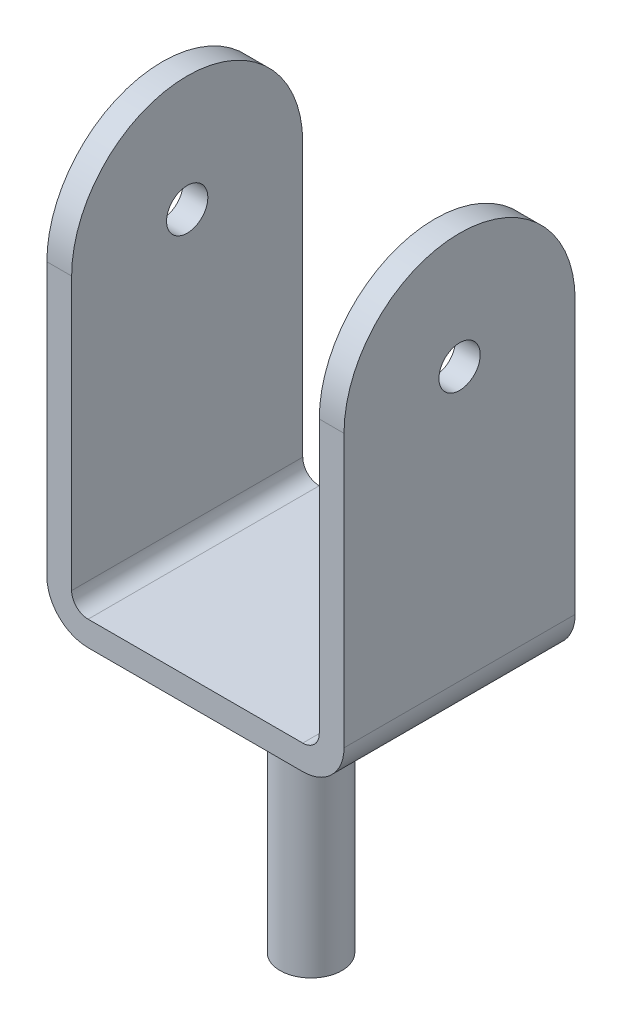
ISO-10303-21;
HEADER;
FILE_DESCRIPTION(('STEP AP214'),'2;1');
FILE_NAME('part.step','',(''),(''),'','','');
FILE_SCHEMA(('AUTOMOTIVE_DESIGN { 1 0 10303 214 1 1 1 1 }'));
ENDSEC;
DATA;
#1=APPLICATION_CONTEXT('core data for automotive mechanical design processes');
#2=APPLICATION_PROTOCOL_DEFINITION('international standard','automotive_design',2000,#1);
#3=PRODUCT_CONTEXT('',#1,'mechanical');
#4=PRODUCT('Part','Part','',(#3));
#5=PRODUCT_RELATED_PRODUCT_CATEGORY('part','',(#4));
#6=PRODUCT_DEFINITION_FORMATION('','',#4);
#7=PRODUCT_DEFINITION_CONTEXT('part definition',#1,'design');
#8=PRODUCT_DEFINITION('design','',#6,#7);
#9=PRODUCT_DEFINITION_SHAPE('','',#8);
#10=(LENGTH_UNIT() NAMED_UNIT(*) SI_UNIT(.MILLI.,.METRE.));
#11=(NAMED_UNIT(*) PLANE_ANGLE_UNIT() SI_UNIT($,.RADIAN.));
#12=(NAMED_UNIT(*) SI_UNIT($,.STERADIAN.) SOLID_ANGLE_UNIT());
#13=UNCERTAINTY_MEASURE_WITH_UNIT(LENGTH_MEASURE(1.E-05),#10,'distance_accuracy_value','');
#14=(GEOMETRIC_REPRESENTATION_CONTEXT(3) GLOBAL_UNCERTAINTY_ASSIGNED_CONTEXT((#13)) GLOBAL_UNIT_ASSIGNED_CONTEXT((#10,
#11,#12)) REPRESENTATION_CONTEXT('',''));
#15=CARTESIAN_POINT('',(0.,0.,0.));
#16=DIRECTION('',(0.,0.,1.));
#17=DIRECTION('',(1.,0.,0.));
#18=AXIS2_PLACEMENT_3D('',#15,#16,#17);
#19=CARTESIAN_POINT('',(-180.,520.,140.));
#20=DIRECTION('',(1.,0.,0.));
#21=DIRECTION('',(0.,0.,-1.));
#22=AXIS2_PLACEMENT_3D('',#19,#20,#21);
#23=PLANE('',#22);
#24=CARTESIAN_POINT('',(-180.,380.,0.));
#25=DIRECTION('',(1.,0.,0.));
#26=DIRECTION('',(0.,0.,-1.));
#27=AXIS2_PLACEMENT_3D('',#24,#25,#26);
#28=CIRCLE('',#27,25.);
#29=CARTESIAN_POINT('',(-180.,380.,-25.));
#30=VERTEX_POINT('',#29);
#31=EDGE_CURVE('E314',#30,#30,#28,.T.);
#32=ORIENTED_EDGE('',*,*,#31,.T.);
#33=EDGE_LOOP('',(#32));
#34=FACE_BOUND('',#33,.T.);
#35=DIRECTION('',(0.,-1.,0.));
#36=VECTOR('',#35,1.);
#37=CARTESIAN_POINT('',(-180.,520.,140.));
#38=LINE('',#37,#36);
#39=CARTESIAN_POINT('',(-180.,380.,140.));
#40=VERTEX_POINT('',#39);
#41=CARTESIAN_POINT('',(-180.,50.0000000000004,140.));
#42=VERTEX_POINT('',#41);
#43=EDGE_CURVE('E183',#40,#42,#38,.T.);
#44=ORIENTED_EDGE('',*,*,#43,.F.);
#45=CARTESIAN_POINT('',(-180.,380.,0.));
#46=DIRECTION('',(1.,0.,0.));
#47=DIRECTION('',(0.,0.,-1.));
#48=AXIS2_PLACEMENT_3D('',#45,#46,#47);
#49=CIRCLE('',#48,140.);
#50=CARTESIAN_POINT('',(-180.,380.,-140.));
#51=VERTEX_POINT('',#50);
#52=EDGE_CURVE('E173',#51,#40,#49,.T.);
#53=ORIENTED_EDGE('',*,*,#52,.F.);
#54=DIRECTION('',(0.,-1.,0.));
#55=VECTOR('',#54,1.);
#56=CARTESIAN_POINT('',(-180.,520.,-140.));
#57=LINE('',#56,#55);
#58=CARTESIAN_POINT('',(-180.,50.0000000000004,-140.));
#59=VERTEX_POINT('',#58);
#60=EDGE_CURVE('E225',#51,#59,#57,.T.);
#61=ORIENTED_EDGE('',*,*,#60,.T.);
#62=DIRECTION('',(0.,0.,-1.));
#63=VECTOR('',#62,1.);
#64=CARTESIAN_POINT('',(-180.,50.0000000000004,140.));
#65=LINE('',#64,#63);
#66=EDGE_CURVE('E192',#42,#59,#65,.T.);
#67=ORIENTED_EDGE('',*,*,#66,.F.);
#68=EDGE_LOOP('',(#44,#53,#61,#67));
#69=FACE_BOUND('',#68,.T.);
#70=ADVANCED_FACE('F87',(#34,#69),#23,.F.);
#71=CARTESIAN_POINT('',(180.,50.0000000000004,140.));
#72=DIRECTION('',(-1.,0.,0.));
#73=DIRECTION('',(0.,0.,1.));
#74=AXIS2_PLACEMENT_3D('',#71,#72,#73);
#75=PLANE('',#74);
#76=CARTESIAN_POINT('',(180.,380.,0.));
#77=DIRECTION('',(1.,0.,0.));
#78=DIRECTION('',(0.,0.,-1.));
#79=AXIS2_PLACEMENT_3D('',#76,#77,#78);
#80=CIRCLE('',#79,25.);
#81=CARTESIAN_POINT('',(180.,380.,-25.));
#82=VERTEX_POINT('',#81);
#83=EDGE_CURVE('E189',#82,#82,#80,.T.);
#84=ORIENTED_EDGE('',*,*,#83,.F.);
#85=EDGE_LOOP('',(#84));
#86=FACE_BOUND('',#85,.T.);
#87=CARTESIAN_POINT('',(180.,380.,0.));
#88=DIRECTION('',(1.,0.,0.));
#89=DIRECTION('',(0.,0.,-1.));
#90=AXIS2_PLACEMENT_3D('',#87,#88,#89);
#91=CIRCLE('',#90,140.);
#92=CARTESIAN_POINT('',(180.,380.,-140.));
#93=VERTEX_POINT('',#92);
#94=CARTESIAN_POINT('',(180.,380.,140.));
#95=VERTEX_POINT('',#94);
#96=EDGE_CURVE('E101',#93,#95,#91,.T.);
#97=ORIENTED_EDGE('',*,*,#96,.T.);
#98=DIRECTION('',(0.,1.,0.));
#99=VECTOR('',#98,1.);
#100=CARTESIAN_POINT('',(180.,50.0000000000004,140.));
#101=LINE('',#100,#99);
#102=CARTESIAN_POINT('',(180.,50.,140.));
#103=VERTEX_POINT('',#102);
#104=EDGE_CURVE('E207',#103,#95,#101,.T.);
#105=ORIENTED_EDGE('',*,*,#104,.F.);
#106=DIRECTION('',(0.,0.,-1.));
#107=VECTOR('',#106,1.);
#108=CARTESIAN_POINT('',(180.,50.,140.));
#109=LINE('',#108,#107);
#110=CARTESIAN_POINT('',(180.,50.,-140.));
#111=VERTEX_POINT('',#110);
#112=EDGE_CURVE('E253',#103,#111,#109,.T.);
#113=ORIENTED_EDGE('',*,*,#112,.T.);
#114=DIRECTION('',(0.,1.,0.));
#115=VECTOR('',#114,1.);
#116=CARTESIAN_POINT('',(180.,50.0000000000004,-140.));
#117=LINE('',#116,#115);
#118=EDGE_CURVE('E226',#111,#93,#117,.T.);
#119=ORIENTED_EDGE('',*,*,#118,.T.);
#120=EDGE_LOOP('',(#97,#105,#113,#119));
#121=FACE_BOUND('',#120,.T.);
#122=ADVANCED_FACE('F267',(#86,#121),#75,.F.);
#123=CARTESIAN_POINT('',(150.,520.,140.));
#124=DIRECTION('',(1.,0.,0.));
#125=DIRECTION('',(0.,1.,0.));
#126=AXIS2_PLACEMENT_3D('',#123,#124,#125);
#127=PLANE('',#126);
#128=CARTESIAN_POINT('',(150.,380.,0.));
#129=DIRECTION('',(1.,0.,0.));
#130=DIRECTION('',(0.,1.,0.));
#131=AXIS2_PLACEMENT_3D('',#128,#129,#130);
#132=CIRCLE('',#131,25.);
#133=CARTESIAN_POINT('',(150.,380.,-25.));
#134=VERTEX_POINT('',#133);
#135=EDGE_CURVE('E310',#134,#134,#132,.T.);
#136=ORIENTED_EDGE('',*,*,#135,.T.);
#137=EDGE_LOOP('',(#136));
#138=FACE_BOUND('',#137,.T.);
#139=DIRECTION('',(0.,-1.,0.));
#140=VECTOR('',#139,1.);
#141=CARTESIAN_POINT('',(150.,520.,140.));
#142=LINE('',#141,#140);
#143=CARTESIAN_POINT('',(150.,380.,140.));
#144=VERTEX_POINT('',#143);
#145=CARTESIAN_POINT('',(150.,50.0000000000001,140.));
#146=VERTEX_POINT('',#145);
#147=EDGE_CURVE('E215',#144,#146,#142,.T.);
#148=ORIENTED_EDGE('',*,*,#147,.F.);
#149=CARTESIAN_POINT('',(150.,380.,0.));
#150=DIRECTION('',(1.,0.,0.));
#151=DIRECTION('',(0.,1.,0.));
#152=AXIS2_PLACEMENT_3D('',#149,#150,#151);
#153=CIRCLE('',#152,140.);
#154=CARTESIAN_POINT('',(150.,380.,-140.));
#155=VERTEX_POINT('',#154);
#156=EDGE_CURVE('E201',#155,#144,#153,.T.);
#157=ORIENTED_EDGE('',*,*,#156,.F.);
#158=DIRECTION('',(0.,-1.,0.));
#159=VECTOR('',#158,1.);
#160=CARTESIAN_POINT('',(150.,520.,-140.));
#161=LINE('',#160,#159);
#162=CARTESIAN_POINT('',(150.,50.0000000000001,-140.));
#163=VERTEX_POINT('',#162);
#164=EDGE_CURVE('E234',#155,#163,#161,.T.);
#165=ORIENTED_EDGE('',*,*,#164,.T.);
#166=DIRECTION('',(0.,0.,-1.));
#167=VECTOR('',#166,1.);
#168=CARTESIAN_POINT('',(150.,50.0000000000001,140.));
#169=LINE('',#168,#167);
#170=EDGE_CURVE('E249',#146,#163,#169,.T.);
#171=ORIENTED_EDGE('',*,*,#170,.F.);
#172=EDGE_LOOP('',(#148,#157,#165,#171));
#173=FACE_BOUND('',#172,.T.);
#174=ADVANCED_FACE('F289',(#138,#173),#127,.F.);
#175=CARTESIAN_POINT('',(-150.,50.0000000000001,140.));
#176=DIRECTION('',(-1.,0.,0.));
#177=DIRECTION('',(0.,-1.,0.));
#178=AXIS2_PLACEMENT_3D('',#175,#176,#177);
#179=PLANE('',#178);
#180=CARTESIAN_POINT('',(-150.,380.,0.));
#181=DIRECTION('',(-1.,0.,0.));
#182=DIRECTION('',(0.,-1.,0.));
#183=AXIS2_PLACEMENT_3D('',#180,#181,#182);
#184=CIRCLE('',#183,25.);
#185=CARTESIAN_POINT('',(-150.,380.,-25.));
#186=VERTEX_POINT('',#185);
#187=EDGE_CURVE('E89',#186,#186,#184,.T.);
#188=ORIENTED_EDGE('',*,*,#187,.T.);
#189=EDGE_LOOP('',(#188));
#190=FACE_BOUND('',#189,.T.);
#191=CARTESIAN_POINT('',(-150.,380.,0.));
#192=DIRECTION('',(-1.,0.,0.));
#193=DIRECTION('',(0.,-1.,0.));
#194=AXIS2_PLACEMENT_3D('',#191,#192,#193);
#195=CIRCLE('',#194,140.);
#196=CARTESIAN_POINT('',(-150.,380.,140.));
#197=VERTEX_POINT('',#196);
#198=CARTESIAN_POINT('',(-150.,380.,-140.));
#199=VERTEX_POINT('',#198);
#200=EDGE_CURVE('E108',#197,#199,#195,.T.);
#201=ORIENTED_EDGE('',*,*,#200,.F.);
#202=DIRECTION('',(0.,1.,0.));
#203=VECTOR('',#202,1.);
#204=CARTESIAN_POINT('',(-150.,50.0000000000001,140.));
#205=LINE('',#204,#203);
#206=CARTESIAN_POINT('',(-150.,50.,140.));
#207=VERTEX_POINT('',#206);
#208=EDGE_CURVE('E188',#207,#197,#205,.T.);
#209=ORIENTED_EDGE('',*,*,#208,.F.);
#210=DIRECTION('',(0.,0.,-1.));
#211=VECTOR('',#210,1.);
#212=CARTESIAN_POINT('',(-150.,50.,140.));
#213=LINE('',#212,#211);
#214=CARTESIAN_POINT('',(-150.,50.,-140.));
#215=VERTEX_POINT('',#214);
#216=EDGE_CURVE('E222',#207,#215,#213,.T.);
#217=ORIENTED_EDGE('',*,*,#216,.T.);
#218=DIRECTION('',(0.,1.,0.));
#219=VECTOR('',#218,1.);
#220=CARTESIAN_POINT('',(-150.,50.0000000000001,-140.));
#221=LINE('',#220,#219);
#222=EDGE_CURVE('E195',#215,#199,#221,.T.);
#223=ORIENTED_EDGE('',*,*,#222,.T.);
#224=EDGE_LOOP('',(#201,#209,#217,#223));
#225=FACE_BOUND('',#224,.T.);
#226=ADVANCED_FACE('F305',(#190,#225),#179,.F.);
#227=CARTESIAN_POINT('',(-130.,50.,140.));
#228=DIRECTION('',(0.,0.,-1.));
#229=DIRECTION('',(-1.,0.,0.));
#230=AXIS2_PLACEMENT_3D('',#227,#228,#229);
#231=CYLINDRICAL_SURFACE('',#230,50.);
#232=CARTESIAN_POINT('',(-130.,50.,-140.));
#233=DIRECTION('',(0.,0.,1.));
#234=DIRECTION('',(1.,0.,0.));
#235=AXIS2_PLACEMENT_3D('',#232,#233,#234);
#236=CIRCLE('',#235,50.);
#237=CARTESIAN_POINT('',(-130.,0.,-140.));
#238=VERTEX_POINT('',#237);
#239=EDGE_CURVE('E221',#59,#238,#236,.T.);
#240=ORIENTED_EDGE('',*,*,#239,.T.);
#241=DIRECTION('',(0.,0.,-1.));
#242=VECTOR('',#241,1.);
#243=CARTESIAN_POINT('',(-130.,0.,140.));
#244=LINE('',#243,#242);
#245=CARTESIAN_POINT('',(-130.,0.,140.));
#246=VERTEX_POINT('',#245);
#247=EDGE_CURVE('E260',#246,#238,#244,.T.);
#248=ORIENTED_EDGE('',*,*,#247,.F.);
#249=CARTESIAN_POINT('',(-130.,50.,140.));
#250=DIRECTION('',(0.,0.,1.));
#251=DIRECTION('',(1.,0.,0.));
#252=AXIS2_PLACEMENT_3D('',#249,#250,#251);
#253=CIRCLE('',#252,50.);
#254=EDGE_CURVE('E193',#42,#246,#253,.T.);
#255=ORIENTED_EDGE('',*,*,#254,.F.);
#256=ORIENTED_EDGE('',*,*,#66,.T.);
#257=EDGE_LOOP('',(#240,#248,#255,#256));
#258=FACE_BOUND('',#257,.T.);
#259=ADVANCED_FACE('F283',(#258),#231,.T.);
#260=CARTESIAN_POINT('',(-130.,0.,140.));
#261=DIRECTION('',(0.,1.,0.));
#262=DIRECTION('',(0.,0.,1.));
#263=AXIS2_PLACEMENT_3D('',#260,#261,#262);
#264=PLANE('',#263);
#265=CARTESIAN_POINT('',(0.,0.,0.));
#266=DIRECTION('',(0.,1.,0.));
#267=DIRECTION('',(0.,0.,1.));
#268=AXIS2_PLACEMENT_3D('',#265,#266,#267);
#269=CIRCLE('',#268,37.5);
#270=CARTESIAN_POINT('',(0.,0.,37.5));
#271=VERTEX_POINT('',#270);
#272=EDGE_CURVE('E320',#271,#271,#269,.T.);
#273=ORIENTED_EDGE('',*,*,#272,.T.);
#274=EDGE_LOOP('',(#273));
#275=FACE_BOUND('',#274,.T.);
#276=DIRECTION('',(1.,0.,0.));
#277=VECTOR('',#276,1.);
#278=CARTESIAN_POINT('',(-130.,0.,-140.));
#279=LINE('',#278,#277);
#280=CARTESIAN_POINT('',(130.,0.,-140.));
#281=VERTEX_POINT('',#280);
#282=EDGE_CURVE('E227',#238,#281,#279,.T.);
#283=ORIENTED_EDGE('',*,*,#282,.T.);
#284=DIRECTION('',(0.,0.,-1.));
#285=VECTOR('',#284,1.);
#286=CARTESIAN_POINT('',(130.,0.,140.));
#287=LINE('',#286,#285);
#288=CARTESIAN_POINT('',(130.,0.,140.));
#289=VERTEX_POINT('',#288);
#290=EDGE_CURVE('E255',#289,#281,#287,.T.);
#291=ORIENTED_EDGE('',*,*,#290,.F.);
#292=DIRECTION('',(1.,0.,0.));
#293=VECTOR('',#292,1.);
#294=CARTESIAN_POINT('',(-130.,0.,140.));
#295=LINE('',#294,#293);
#296=EDGE_CURVE('E197',#246,#289,#295,.T.);
#297=ORIENTED_EDGE('',*,*,#296,.F.);
#298=ORIENTED_EDGE('',*,*,#247,.T.);
#299=EDGE_LOOP('',(#283,#291,#297,#298));
#300=FACE_BOUND('',#299,.T.);
#301=ADVANCED_FACE('F276',(#275,#300),#264,.F.);
#302=CARTESIAN_POINT('',(130.,50.,140.));
#303=DIRECTION('',(0.,0.,-1.));
#304=DIRECTION('',(-1.,0.,0.));
#305=AXIS2_PLACEMENT_3D('',#302,#303,#304);
#306=CYLINDRICAL_SURFACE('',#305,50.);
#307=CARTESIAN_POINT('',(130.,50.,-140.));
#308=DIRECTION('',(0.,0.,1.));
#309=DIRECTION('',(1.,0.,0.));
#310=AXIS2_PLACEMENT_3D('',#307,#308,#309);
#311=CIRCLE('',#310,50.);
#312=EDGE_CURVE('E228',#281,#111,#311,.T.);
#313=ORIENTED_EDGE('',*,*,#312,.T.);
#314=ORIENTED_EDGE('',*,*,#112,.F.);
#315=CARTESIAN_POINT('',(130.,50.,140.));
#316=DIRECTION('',(0.,0.,1.));
#317=DIRECTION('',(1.,0.,0.));
#318=AXIS2_PLACEMENT_3D('',#315,#316,#317);
#319=CIRCLE('',#318,50.);
#320=EDGE_CURVE('E210',#289,#103,#319,.T.);
#321=ORIENTED_EDGE('',*,*,#320,.F.);
#322=ORIENTED_EDGE('',*,*,#290,.T.);
#323=EDGE_LOOP('',(#313,#314,#321,#322));
#324=FACE_BOUND('',#323,.T.);
#325=ADVANCED_FACE('F273',(#324),#306,.T.);
#326=CARTESIAN_POINT('',(130.,50.,140.));
#327=DIRECTION('',(0.,0.,-1.));
#328=DIRECTION('',(-1.,0.,0.));
#329=AXIS2_PLACEMENT_3D('',#326,#327,#328);
#330=CYLINDRICAL_SURFACE('',#329,20.);
#331=CARTESIAN_POINT('',(130.,50.,-140.));
#332=DIRECTION('',(0.,0.,-1.));
#333=DIRECTION('',(-1.,0.,0.));
#334=AXIS2_PLACEMENT_3D('',#331,#332,#333);
#335=CIRCLE('',#334,20.);
#336=CARTESIAN_POINT('',(130.,30.,-140.));
#337=VERTEX_POINT('',#336);
#338=EDGE_CURVE('E235',#163,#337,#335,.T.);
#339=ORIENTED_EDGE('',*,*,#338,.T.);
#340=DIRECTION('',(0.,0.,-1.));
#341=VECTOR('',#340,1.);
#342=CARTESIAN_POINT('',(130.,30.,140.));
#343=LINE('',#342,#341);
#344=CARTESIAN_POINT('',(130.,30.,140.));
#345=VERTEX_POINT('',#344);
#346=EDGE_CURVE('E241',#345,#337,#343,.T.);
#347=ORIENTED_EDGE('',*,*,#346,.F.);
#348=CARTESIAN_POINT('',(130.,50.,140.));
#349=DIRECTION('',(0.,0.,-1.));
#350=DIRECTION('',(-1.,0.,0.));
#351=AXIS2_PLACEMENT_3D('',#348,#349,#350);
#352=CIRCLE('',#351,20.);
#353=EDGE_CURVE('E212',#146,#345,#352,.T.);
#354=ORIENTED_EDGE('',*,*,#353,.F.);
#355=ORIENTED_EDGE('',*,*,#170,.T.);
#356=EDGE_LOOP('',(#339,#347,#354,#355));
#357=FACE_BOUND('',#356,.T.);
#358=ADVANCED_FACE('F295',(#357),#330,.F.);
#359=CARTESIAN_POINT('',(130.,30.,140.));
#360=DIRECTION('',(0.,-1.,0.));
#361=DIRECTION('',(0.,0.,-1.));
#362=AXIS2_PLACEMENT_3D('',#359,#360,#361);
#363=PLANE('',#362);
#364=DIRECTION('',(-1.,0.,0.));
#365=VECTOR('',#364,1.);
#366=CARTESIAN_POINT('',(130.,30.,-140.));
#367=LINE('',#366,#365);
#368=CARTESIAN_POINT('',(-130.,30.,-140.));
#369=VERTEX_POINT('',#368);
#370=EDGE_CURVE('E240',#337,#369,#367,.T.);
#371=ORIENTED_EDGE('',*,*,#370,.T.);
#372=DIRECTION('',(0.,0.,-1.));
#373=VECTOR('',#372,1.);
#374=CARTESIAN_POINT('',(-130.,30.,140.));
#375=LINE('',#374,#373);
#376=CARTESIAN_POINT('',(-130.,30.,140.));
#377=VERTEX_POINT('',#376);
#378=EDGE_CURVE('E245',#377,#369,#375,.T.);
#379=ORIENTED_EDGE('',*,*,#378,.F.);
#380=DIRECTION('',(-1.,0.,0.));
#381=VECTOR('',#380,1.);
#382=CARTESIAN_POINT('',(130.,30.,140.));
#383=LINE('',#382,#381);
#384=EDGE_CURVE('E216',#345,#377,#383,.T.);
#385=ORIENTED_EDGE('',*,*,#384,.F.);
#386=ORIENTED_EDGE('',*,*,#346,.T.);
#387=EDGE_LOOP('',(#371,#379,#385,#386));
#388=FACE_BOUND('',#387,.T.);
#389=ADVANCED_FACE('F298',(#388),#363,.F.);
#390=CARTESIAN_POINT('',(-130.,50.,140.));
#391=DIRECTION('',(0.,0.,-1.));
#392=DIRECTION('',(-1.,0.,0.));
#393=AXIS2_PLACEMENT_3D('',#390,#391,#392);
#394=CYLINDRICAL_SURFACE('',#393,20.);
#395=CARTESIAN_POINT('',(-130.,50.,-140.));
#396=DIRECTION('',(0.,0.,-1.));
#397=DIRECTION('',(-1.,0.,0.));
#398=AXIS2_PLACEMENT_3D('',#395,#396,#397);
#399=CIRCLE('',#398,20.);
#400=EDGE_CURVE('E199',#369,#215,#399,.T.);
#401=ORIENTED_EDGE('',*,*,#400,.T.);
#402=ORIENTED_EDGE('',*,*,#216,.F.);
#403=CARTESIAN_POINT('',(-130.,50.,140.));
#404=DIRECTION('',(0.,0.,-1.));
#405=DIRECTION('',(-1.,0.,0.));
#406=AXIS2_PLACEMENT_3D('',#403,#404,#405);
#407=CIRCLE('',#406,20.);
#408=EDGE_CURVE('E217',#377,#207,#407,.T.);
#409=ORIENTED_EDGE('',*,*,#408,.F.);
#410=ORIENTED_EDGE('',*,*,#378,.T.);
#411=EDGE_LOOP('',(#401,#402,#409,#410));
#412=FACE_BOUND('',#411,.T.);
#413=ADVANCED_FACE('F302',(#412),#394,.F.);
#414=CARTESIAN_POINT('',(-130.,50.,140.));
#415=DIRECTION('',(0.,0.,1.));
#416=DIRECTION('',(1.,0.,0.));
#417=AXIS2_PLACEMENT_3D('',#414,#415,#416);
#418=PLANE('',#417);
#419=DIRECTION('',(1.,0.,0.));
#420=VECTOR('',#419,1.);
#421=CARTESIAN_POINT('',(-180.,380.,140.));
#422=LINE('',#421,#420);
#423=EDGE_CURVE('E176',#40,#197,#422,.T.);
#424=ORIENTED_EDGE('',*,*,#423,.F.);
#425=ORIENTED_EDGE('',*,*,#43,.T.);
#426=ORIENTED_EDGE('',*,*,#254,.T.);
#427=ORIENTED_EDGE('',*,*,#296,.T.);
#428=ORIENTED_EDGE('',*,*,#320,.T.);
#429=ORIENTED_EDGE('',*,*,#104,.T.);
#430=DIRECTION('',(1.,0.,0.));
#431=VECTOR('',#430,1.);
#432=CARTESIAN_POINT('',(-180.,380.,140.));
#433=LINE('',#432,#431);
#434=EDGE_CURVE('E12',#144,#95,#433,.T.);
#435=ORIENTED_EDGE('',*,*,#434,.F.);
#436=ORIENTED_EDGE('',*,*,#147,.T.);
#437=ORIENTED_EDGE('',*,*,#353,.T.);
#438=ORIENTED_EDGE('',*,*,#384,.T.);
#439=ORIENTED_EDGE('',*,*,#408,.T.);
#440=ORIENTED_EDGE('',*,*,#208,.T.);
#441=EDGE_LOOP('',(#424,#425,#426,#427,#428,#429,#435,#436,#437,#438,#439,#440));
#442=FACE_BOUND('',#441,.T.);
#443=ADVANCED_FACE('F184',(#442),#418,.T.);
#444=CARTESIAN_POINT('',(-130.,50.,-140.));
#445=DIRECTION('',(0.,0.,1.));
#446=DIRECTION('',(1.,0.,0.));
#447=AXIS2_PLACEMENT_3D('',#444,#445,#446);
#448=PLANE('',#447);
#449=ORIENTED_EDGE('',*,*,#60,.F.);
#450=DIRECTION('',(1.,0.,0.));
#451=VECTOR('',#450,1.);
#452=CARTESIAN_POINT('',(-180.,380.,-140.));
#453=LINE('',#452,#451);
#454=EDGE_CURVE('E179',#51,#199,#453,.T.);
#455=ORIENTED_EDGE('',*,*,#454,.T.);
#456=ORIENTED_EDGE('',*,*,#222,.F.);
#457=ORIENTED_EDGE('',*,*,#400,.F.);
#458=ORIENTED_EDGE('',*,*,#370,.F.);
#459=ORIENTED_EDGE('',*,*,#338,.F.);
#460=ORIENTED_EDGE('',*,*,#164,.F.);
#461=DIRECTION('',(1.,0.,0.));
#462=VECTOR('',#461,1.);
#463=CARTESIAN_POINT('',(-180.,380.,-140.));
#464=LINE('',#463,#462);
#465=EDGE_CURVE('E92',#155,#93,#464,.T.);
#466=ORIENTED_EDGE('',*,*,#465,.T.);
#467=ORIENTED_EDGE('',*,*,#118,.F.);
#468=ORIENTED_EDGE('',*,*,#312,.F.);
#469=ORIENTED_EDGE('',*,*,#282,.F.);
#470=ORIENTED_EDGE('',*,*,#239,.F.);
#471=EDGE_LOOP('',(#449,#455,#456,#457,#458,#459,#460,#466,#467,#468,#469,#470));
#472=FACE_BOUND('',#471,.T.);
#473=ADVANCED_FACE('F262',(#472),#448,.F.);
#474=CARTESIAN_POINT('',(-180.,380.,0.));
#475=DIRECTION('',(1.,0.,0.));
#476=DIRECTION('',(0.,0.,-1.));
#477=AXIS2_PLACEMENT_3D('',#474,#475,#476);
#478=CYLINDRICAL_SURFACE('',#477,140.);
#479=ORIENTED_EDGE('',*,*,#156,.T.);
#480=ORIENTED_EDGE('',*,*,#434,.T.);
#481=ORIENTED_EDGE('',*,*,#96,.F.);
#482=ORIENTED_EDGE('',*,*,#465,.F.);
#483=EDGE_LOOP('',(#479,#480,#481,#482));
#484=FACE_BOUND('',#483,.T.);
#485=ADVANCED_FACE('F416',(#484),#478,.T.);
#486=ORIENTED_EDGE('',*,*,#200,.T.);
#487=ORIENTED_EDGE('',*,*,#454,.F.);
#488=ORIENTED_EDGE('',*,*,#52,.T.);
#489=ORIENTED_EDGE('',*,*,#423,.T.);
#490=EDGE_LOOP('',(#486,#487,#488,#489));
#491=FACE_BOUND('',#490,.T.);
#492=ADVANCED_FACE('F171',(#491),#478,.T.);
#493=CARTESIAN_POINT('',(-180.,380.,0.));
#494=DIRECTION('',(1.,0.,0.));
#495=DIRECTION('',(0.,0.,-1.));
#496=AXIS2_PLACEMENT_3D('',#493,#494,#495);
#497=CYLINDRICAL_SURFACE('',#496,25.);
#498=CARTESIAN_POINT('',(-180.,380.,-25.));
#499=CARTESIAN_POINT('',(-179.6875,380.,-25.));
#500=CARTESIAN_POINT('',(-179.375,380.,-25.));
#501=CARTESIAN_POINT('',(-178.75,380.,-25.));
#502=CARTESIAN_POINT('',(-178.4375,380.,-25.));
#503=CARTESIAN_POINT('',(-177.8125,380.,-25.));
#504=CARTESIAN_POINT('',(-177.5,380.,-25.));
#505=CARTESIAN_POINT('',(-176.875,380.,-25.));
#506=CARTESIAN_POINT('',(-176.5625,380.,-25.));
#507=CARTESIAN_POINT('',(-175.9375,380.,-25.));
#508=CARTESIAN_POINT('',(-175.625,380.,-25.));
#509=CARTESIAN_POINT('',(-175.,380.,-25.));
#510=CARTESIAN_POINT('',(-174.6875,380.,-25.));
#511=CARTESIAN_POINT('',(-174.0625,380.,-25.));
#512=CARTESIAN_POINT('',(-173.75,380.,-25.));
#513=CARTESIAN_POINT('',(-173.125,380.,-25.));
#514=CARTESIAN_POINT('',(-172.8125,380.,-25.));
#515=CARTESIAN_POINT('',(-172.1875,380.,-25.));
#516=CARTESIAN_POINT('',(-171.875,380.,-25.));
#517=CARTESIAN_POINT('',(-171.25,380.,-25.));
#518=CARTESIAN_POINT('',(-170.9375,380.,-25.));
#519=CARTESIAN_POINT('',(-170.3125,380.,-25.));
#520=CARTESIAN_POINT('',(-170.,380.,-25.));
#521=CARTESIAN_POINT('',(-169.375,380.,-25.));
#522=CARTESIAN_POINT('',(-169.0625,380.,-25.));
#523=CARTESIAN_POINT('',(-168.4375,380.,-25.));
#524=CARTESIAN_POINT('',(-168.125,380.,-25.));
#525=CARTESIAN_POINT('',(-167.5,380.,-25.));
#526=CARTESIAN_POINT('',(-167.1875,380.,-25.));
#527=CARTESIAN_POINT('',(-166.5625,380.,-25.));
#528=CARTESIAN_POINT('',(-166.25,380.,-25.));
#529=CARTESIAN_POINT('',(-165.625,380.,-25.));
#530=CARTESIAN_POINT('',(-165.3125,380.,-25.));
#531=CARTESIAN_POINT('',(-164.6875,380.,-25.));
#532=CARTESIAN_POINT('',(-164.375,380.,-25.));
#533=CARTESIAN_POINT('',(-163.75,380.,-25.));
#534=CARTESIAN_POINT('',(-163.4375,380.,-25.));
#535=CARTESIAN_POINT('',(-162.8125,380.,-25.));
#536=CARTESIAN_POINT('',(-162.5,380.,-25.));
#537=CARTESIAN_POINT('',(-161.875,380.,-25.));
#538=CARTESIAN_POINT('',(-161.5625,380.,-25.));
#539=CARTESIAN_POINT('',(-160.9375,380.,-25.));
#540=CARTESIAN_POINT('',(-160.625,380.,-25.));
#541=CARTESIAN_POINT('',(-160.,380.,-25.));
#542=CARTESIAN_POINT('',(-159.6875,380.,-25.));
#543=CARTESIAN_POINT('',(-159.0625,380.,-25.));
#544=CARTESIAN_POINT('',(-158.75,380.,-25.));
#545=CARTESIAN_POINT('',(-158.125,380.,-25.));
#546=CARTESIAN_POINT('',(-157.8125,380.,-25.));
#547=CARTESIAN_POINT('',(-157.1875,380.,-25.));
#548=CARTESIAN_POINT('',(-156.875,380.,-25.));
#549=CARTESIAN_POINT('',(-156.25,380.,-25.));
#550=CARTESIAN_POINT('',(-155.9375,380.,-25.));
#551=CARTESIAN_POINT('',(-155.3125,380.,-25.));
#552=CARTESIAN_POINT('',(-155.,380.,-25.));
#553=CARTESIAN_POINT('',(-154.375,380.,-25.));
#554=CARTESIAN_POINT('',(-154.0625,380.,-25.));
#555=CARTESIAN_POINT('',(-153.4375,380.,-25.));
#556=CARTESIAN_POINT('',(-153.125,380.,-25.));
#557=CARTESIAN_POINT('',(-152.5,380.,-25.));
#558=CARTESIAN_POINT('',(-152.1875,380.,-25.));
#559=CARTESIAN_POINT('',(-151.5625,380.,-25.));
#560=CARTESIAN_POINT('',(-151.25,380.,-25.));
#561=CARTESIAN_POINT('',(-150.625,380.,-25.));
#562=CARTESIAN_POINT('',(-150.3125,380.,-25.));
#563=CARTESIAN_POINT('',(-150.,380.,-25.));
#564=B_SPLINE_CURVE_WITH_KNOTS('',3,(#498,#499,#500,#501,#502,#503,#504,#505,#506,#507,#508,
#509,#510,#511,#512,#513,#514,#515,#516,#517,#518,#519,#520,#521,#522,#523,#524,#525,#526,#527,
#528,#529,#530,#531,#532,#533,#534,#535,#536,#537,#538,#539,#540,#541,#542,#543,#544,#545,#546,
#547,#548,#549,#550,#551,#552,#553,#554,#555,#556,#557,#558,#559,#560,#561,#562,#563),
.UNSPECIFIED.,.F.,.F.,(4,2,2,2,2,2,2,2,2,2,2,2,2,2,2,2,2,2,2,2,2,2,2,2,2,2,2,2,2,2,2,2,4),(0.,
0.937500000000008,1.87500000000002,2.81250000000002,3.75,4.68750000000001,5.62500000000002,
6.56250000000003,7.50000000000001,8.43750000000001,9.37500000000002,10.3125,11.25,12.1875,
13.125,14.0625,15.,15.9375,16.875,17.8125,18.75,19.6875,20.625,21.5625,22.5,23.4375,24.375,
25.3125,26.25,27.1875,28.125,29.0625,30.),.UNSPECIFIED.);
#565=EDGE_CURVE('BSEAM345',#30,#186,#564,.T.);
#566=ORIENTED_EDGE('',*,*,#31,.F.);
#567=ORIENTED_EDGE('',*,*,#187,.F.);
#568=ORIENTED_EDGE('',*,*,#565,.T.);
#569=ORIENTED_EDGE('',*,*,#565,.F.);
#570=EDGE_LOOP('',(#566,#568,#567,#569));
#571=FACE_BOUND('',#570,.T.);
#572=ADVANCED_FACE('F345',(#571),#497,.F.);
#573=CARTESIAN_POINT('',(180.,380.,-25.));
#574=CARTESIAN_POINT('',(179.6875,380.,-25.));
#575=CARTESIAN_POINT('',(179.375,380.,-25.));
#576=CARTESIAN_POINT('',(178.75,380.,-25.));
#577=CARTESIAN_POINT('',(178.4375,380.,-25.));
#578=CARTESIAN_POINT('',(177.8125,380.,-25.));
#579=CARTESIAN_POINT('',(177.5,380.,-25.));
#580=CARTESIAN_POINT('',(176.875,380.,-25.));
#581=CARTESIAN_POINT('',(176.5625,380.,-25.));
#582=CARTESIAN_POINT('',(175.9375,380.,-25.));
#583=CARTESIAN_POINT('',(175.625,380.,-25.));
#584=CARTESIAN_POINT('',(175.,380.,-25.));
#585=CARTESIAN_POINT('',(174.6875,380.,-25.));
#586=CARTESIAN_POINT('',(174.0625,380.,-25.));
#587=CARTESIAN_POINT('',(173.75,380.,-25.));
#588=CARTESIAN_POINT('',(173.125,380.,-25.));
#589=CARTESIAN_POINT('',(172.8125,380.,-25.));
#590=CARTESIAN_POINT('',(172.1875,380.,-25.));
#591=CARTESIAN_POINT('',(171.875,380.,-25.));
#592=CARTESIAN_POINT('',(171.25,380.,-25.));
#593=CARTESIAN_POINT('',(170.9375,380.,-25.));
#594=CARTESIAN_POINT('',(170.3125,380.,-25.));
#595=CARTESIAN_POINT('',(170.,380.,-25.));
#596=CARTESIAN_POINT('',(169.375,380.,-25.));
#597=CARTESIAN_POINT('',(169.0625,380.,-25.));
#598=CARTESIAN_POINT('',(168.4375,380.,-25.));
#599=CARTESIAN_POINT('',(168.125,380.,-25.));
#600=CARTESIAN_POINT('',(167.5,380.,-25.));
#601=CARTESIAN_POINT('',(167.1875,380.,-25.));
#602=CARTESIAN_POINT('',(166.5625,380.,-25.));
#603=CARTESIAN_POINT('',(166.25,380.,-25.));
#604=CARTESIAN_POINT('',(165.625,380.,-25.));
#605=CARTESIAN_POINT('',(165.3125,380.,-25.));
#606=CARTESIAN_POINT('',(164.6875,380.,-25.));
#607=CARTESIAN_POINT('',(164.375,380.,-25.));
#608=CARTESIAN_POINT('',(163.75,380.,-25.));
#609=CARTESIAN_POINT('',(163.4375,380.,-25.));
#610=CARTESIAN_POINT('',(162.8125,380.,-25.));
#611=CARTESIAN_POINT('',(162.5,380.,-25.));
#612=CARTESIAN_POINT('',(161.875,380.,-25.));
#613=CARTESIAN_POINT('',(161.5625,380.,-25.));
#614=CARTESIAN_POINT('',(160.9375,380.,-25.));
#615=CARTESIAN_POINT('',(160.625,380.,-25.));
#616=CARTESIAN_POINT('',(160.,380.,-25.));
#617=CARTESIAN_POINT('',(159.6875,380.,-25.));
#618=CARTESIAN_POINT('',(159.0625,380.,-25.));
#619=CARTESIAN_POINT('',(158.75,380.,-25.));
#620=CARTESIAN_POINT('',(158.125,380.,-25.));
#621=CARTESIAN_POINT('',(157.8125,380.,-25.));
#622=CARTESIAN_POINT('',(157.1875,380.,-25.));
#623=CARTESIAN_POINT('',(156.875,380.,-25.));
#624=CARTESIAN_POINT('',(156.25,380.,-25.));
#625=CARTESIAN_POINT('',(155.9375,380.,-25.));
#626=CARTESIAN_POINT('',(155.3125,380.,-25.));
#627=CARTESIAN_POINT('',(155.,380.,-25.));
#628=CARTESIAN_POINT('',(154.375,380.,-25.));
#629=CARTESIAN_POINT('',(154.0625,380.,-25.));
#630=CARTESIAN_POINT('',(153.4375,380.,-25.));
#631=CARTESIAN_POINT('',(153.125,380.,-25.));
#632=CARTESIAN_POINT('',(152.5,380.,-25.));
#633=CARTESIAN_POINT('',(152.1875,380.,-25.));
#634=CARTESIAN_POINT('',(151.5625,380.,-25.));
#635=CARTESIAN_POINT('',(151.25,380.,-25.));
#636=CARTESIAN_POINT('',(150.625,380.,-25.));
#637=CARTESIAN_POINT('',(150.3125,380.,-25.));
#638=CARTESIAN_POINT('',(150.,380.,-25.));
#639=B_SPLINE_CURVE_WITH_KNOTS('',3,(#573,#574,#575,#576,#577,#578,#579,#580,#581,#582,#583,
#584,#585,#586,#587,#588,#589,#590,#591,#592,#593,#594,#595,#596,#597,#598,#599,#600,#601,#602,
#603,#604,#605,#606,#607,#608,#609,#610,#611,#612,#613,#614,#615,#616,#617,#618,#619,#620,#621,
#622,#623,#624,#625,#626,#627,#628,#629,#630,#631,#632,#633,#634,#635,#636,#637,#638),
.UNSPECIFIED.,.F.,.F.,(4,2,2,2,2,2,2,2,2,2,2,2,2,2,2,2,2,2,2,2,2,2,2,2,2,2,2,2,2,2,2,2,4),(0.,
0.93749999999998,1.87500000000002,2.8125,3.75000000000003,4.68750000000001,5.62499999999999,
6.56250000000003,7.50000000000001,8.43749999999999,9.37500000000002,10.3125,11.25,12.1875,
13.125,14.0625,15.,15.9375,16.875,17.8125,18.75,19.6875,20.625,21.5625,22.5,23.4375,24.375,
25.3125,26.25,27.1875,28.125,29.0625,30.),.UNSPECIFIED.);
#640=EDGE_CURVE('BSEAM334',#82,#134,#639,.T.);
#641=ORIENTED_EDGE('',*,*,#83,.T.);
#642=ORIENTED_EDGE('',*,*,#135,.F.);
#643=ORIENTED_EDGE('',*,*,#640,.T.);
#644=ORIENTED_EDGE('',*,*,#640,.F.);
#645=EDGE_LOOP('',(#641,#643,#642,#644));
#646=FACE_BOUND('',#645,.T.);
#647=ADVANCED_FACE('F334',(#646),#497,.F.);
#648=CARTESIAN_POINT('',(0.,-325.,0.));
#649=DIRECTION('',(0.,1.,0.));
#650=DIRECTION('',(0.,0.,1.));
#651=AXIS2_PLACEMENT_3D('',#648,#649,#650);
#652=CYLINDRICAL_SURFACE('',#651,37.5);
#653=CARTESIAN_POINT('',(0.,-325.,0.));
#654=DIRECTION('',(0.,1.,0.));
#655=DIRECTION('',(0.,0.,1.));
#656=AXIS2_PLACEMENT_3D('',#653,#654,#655);
#657=CIRCLE('',#656,37.5);
#658=CARTESIAN_POINT('',(0.,-325.,37.5));
#659=VERTEX_POINT('',#658);
#660=EDGE_CURVE('E319',#659,#659,#657,.T.);
#661=ORIENTED_EDGE('',*,*,#660,.T.);
#662=EDGE_LOOP('',(#661));
#663=FACE_BOUND('',#662,.T.);
#664=ORIENTED_EDGE('',*,*,#272,.F.);
#665=EDGE_LOOP('',(#664));
#666=FACE_BOUND('',#665,.T.);
#667=ADVANCED_FACE('F322',(#663,#666),#652,.T.);
#668=CARTESIAN_POINT('',(0.,-325.,0.));
#669=DIRECTION('',(0.,1.,0.));
#670=DIRECTION('',(0.,0.,1.));
#671=AXIS2_PLACEMENT_3D('',#668,#669,#670);
#672=PLANE('',#671);
#673=ORIENTED_EDGE('',*,*,#660,.F.);
#674=EDGE_LOOP('',(#673));
#675=FACE_BOUND('',#674,.T.);
#676=ADVANCED_FACE('F330',(#675),#672,.F.);
#677=CLOSED_SHELL('',(#70,#122,#174,#226,#259,#301,#325,#358,#389,#413,#443,#473,#485,#492,#572,
#647,#667,#676));
#678=MANIFOLD_SOLID_BREP('B2',#677);
#679=ADVANCED_BREP_SHAPE_REPRESENTATION('',(#18,#678),#14);
#680=SHAPE_DEFINITION_REPRESENTATION(#9,#679);
ENDSEC;
END-ISO-10303-21;
